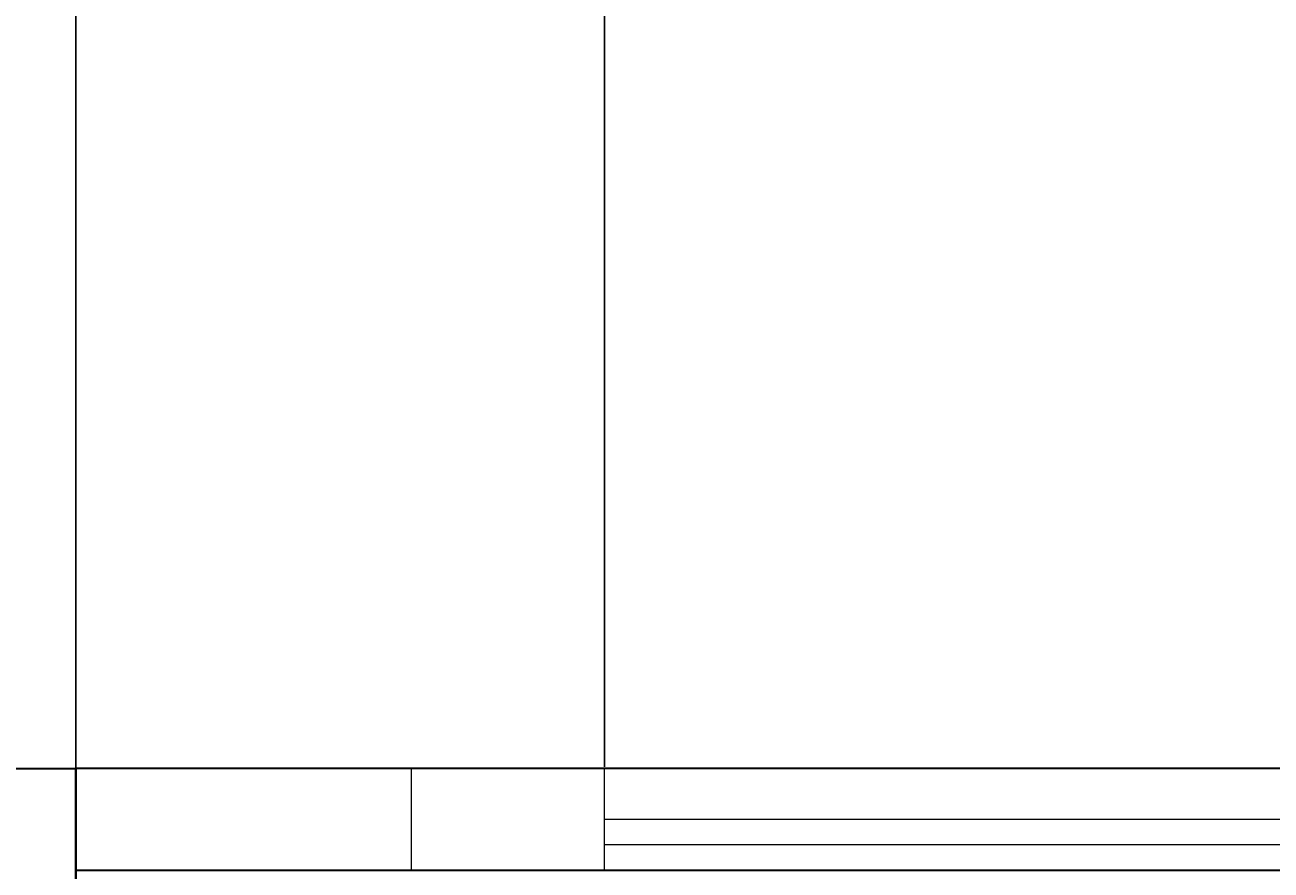
# Model space of a CAD drawing. Units: feet. Extents: x 105 to 1094, y -88 to 588.
# Tile 46 of 59: x 551 to 600, y 437 to 470. Entities that reach past the tile are written whole.
import ezdxf

# ---------------------------------------------------------------- set-up
doc = ezdxf.new("R2010")
doc.units = ezdxf.units.FT
doc.header["$MEASUREMENT"] = 0
for name, color, linetype, lineweight in [('A-ANNO-DIMS', 2, 'Continuous', 18), ('A-FLOR-PROJ', 8, 'Continuous', 25), ('A-GLAZ', 4, 'Continuous', 18), ('A-WALL', 7, 'Continuous', 35)]:
    doc.layers.add(name, color=color, linetype=linetype, lineweight=lineweight)
doc.styles.get("Standard").update_dxf_attribs({"font": 'arial.ttf'})
doc.dimstyles.get("Standard").update_dxf_attribs({"dimtxt": 0.18, "dimasz": 0.18, "dimexe": 0.18, "dimexo": 0.0625, "dimgap": 0.09, "dimtad": 0, "dimtih": 1, "dimtoh": 1, "dimdec": 4, "dimzin": 0, "dimdsep": 46, "dimtxsty": 'Standard', "dimcen": 0.09, "dimadec": 0, "dimazin": 0, "dimtfac": 1, "dimtdec": 4, "dimtofl": 0, "dimtmove": 0, "dimatfit": 3, "dimfxl": 1, "dimtolj": 1, "dimtzin": 0, "dimarcsym": 0})

# ---------------------------------------------------------------- blocks, each defined once
blk = doc.blocks.new('*D21')
at = {"layer": 'A-ANNO-DIMS', "color": 0, "lineweight": -2, "transparency": 16777216}
for p, q in [((849.626, 543.081), (105.458, 543.081)), ((105.638, 542.901), (105.638, 250.263)), ((105.638, -42.739), (105.638, 249.899)), ((849.626, -42.919), (105.458, -42.919))]:
    blk.add_line(p, q, dxfattribs=at)
at = {"layer": 'A-ANNO-DIMS', "color": 0, "transparency": 16777216}
for points in [[(105.608, 542.901), (105.668, 542.901), (105.638, 543.081)], [(105.608, -42.739), (105.668, -42.739), (105.638, -42.919)]]:
    blk.add_solid(points, dxfattribs=at)
at = {"layer": 'Defpoints', "color": 0, "transparency": 16777216}
for p in [(105.638, 543.081), (849.688, 543.081), (849.688, -42.919)]:
    blk.add_point(p, dxfattribs=at)
at = {"layer": 'A-ANNO-DIMS', "color": 0, "transparency": 16777216, "insert": (105.638, 250.081), "char_height": 0.18, "attachment_point": 5}
blk.add_mtext('\\A1;586', dxfattribs=at)
blk = doc.blocks.new('*D32')
at = {"layer": 'A-ANNO-DIMS', "color": 0, "lineweight": -2, "transparency": 16777216}
for p, q in [((646.626, 471.081), (105.458, 471.081)), ((105.638, 470.901), (105.638, 456.263)), ((105.638, 441.261), (105.638, 455.899)), ((646.626, 441.081), (105.458, 441.081))]:
    blk.add_line(p, q, dxfattribs=at)
at = {"layer": 'A-ANNO-DIMS', "color": 0, "transparency": 16777216}
for points in [[(105.608, 470.901), (105.668, 470.901), (105.638, 471.081)], [(105.608, 441.261), (105.668, 441.261), (105.638, 441.081)]]:
    blk.add_solid(points, dxfattribs=at)
at = {"layer": 'Defpoints', "color": 0, "transparency": 16777216}
for p in [(105.638, 471.081), (646.688, 471.081), (646.688, 441.081)]:
    blk.add_point(p, dxfattribs=at)
at = {"layer": 'A-ANNO-DIMS', "color": 0, "transparency": 16777216, "insert": (105.638, 456.081), "char_height": 0.18, "attachment_point": 5}
blk.add_mtext('\\A1;30', dxfattribs=at)
blk = doc.blocks.new('*D47')
at = {"layer": 'A-ANNO-DIMS', "color": 0, "lineweight": -2, "transparency": 16777216}
for p, q in [((552.688, 441.144), (552.688, 588.311)), ((552.868, 588.131), (562.621, 588.131)), ((573.303, 588.131), (563.55, 588.131)), ((573.483, 441.144), (573.483, 588.311))]:
    blk.add_line(p, q, dxfattribs=at)
at = {"layer": 'A-ANNO-DIMS', "color": 0, "transparency": 16777216}
for points in [[(552.868, 588.161), (552.868, 588.101), (552.688, 588.131)], [(573.303, 588.161), (573.303, 588.101), (573.483, 588.131)]]:
    blk.add_solid(points, dxfattribs=at)
at = {"layer": 'Defpoints', "color": 0, "transparency": 16777216}
for p in [(573.483, 588.131), (552.688, 441.081), (573.483, 441.081)]:
    blk.add_point(p, dxfattribs=at)
at = {"layer": 'A-ANNO-DIMS', "color": 0, "transparency": 16777216, "insert": (563.085, 588.131), "char_height": 0.18, "attachment_point": 5}
blk.add_mtext('\\A1;20.794', dxfattribs=at)
blk = doc.blocks.new('*D48')
at = {"layer": 'A-ANNO-DIMS', "color": 0, "lineweight": -2, "transparency": 16777216}
for p, q in [((573.483, 441.144), (573.483, 588.311)), ((573.663, 588.131), (603.263, 588.131)), ((633.303, 588.131), (603.702, 588.131)), ((633.483, 441.144), (633.483, 588.311))]:
    blk.add_line(p, q, dxfattribs=at)
at = {"layer": 'A-ANNO-DIMS', "color": 0, "transparency": 16777216}
for points in [[(573.663, 588.161), (573.663, 588.101), (573.483, 588.131)], [(633.303, 588.161), (633.303, 588.101), (633.483, 588.131)]]:
    blk.add_solid(points, dxfattribs=at)
at = {"layer": 'Defpoints', "color": 0, "transparency": 16777216}
for p in [(633.483, 588.131), (573.483, 441.081), (633.483, 441.081)]:
    blk.add_point(p, dxfattribs=at)
at = {"layer": 'A-ANNO-DIMS', "color": 0, "transparency": 16777216, "insert": (603.483, 588.131), "char_height": 0.18, "attachment_point": 5}
blk.add_mtext('\\A1;60', dxfattribs=at)

msp = doc.modelspace()

# ---------------------------------------------------------------- linework, layer by layer
at = {"layer": 'A-FLOR-PROJ'}
msp.add_line((552.6883, 471.0812), (552.6883, 441.0812), dxfattribs=at)
at = {"layer": 'A-GLAZ'}
for p, q in [((565.8941, 437.0812), (565.8941, 441.0812)), ((573.4826, 437.0812), (573.4826, 441.0812)), ((573.4826, 439.0812), (633.4826, 439.0812)), ((573.4826, 438.0812), (603.4826, 438.0812))]:
    msp.add_line(p, q, dxfattribs=at)
at = {"layer": 'A-WALL'}
for p, q in [((438.6883, 441.0812), (552.6883, 441.0812)), ((552.6883, 295.0812), (552.6883, 441.0812)), ((646.6883, 441.0812), (552.6883, 441.0812)), ((552.6883, 441.0812), (552.6883, 288.0812)), ((552.6883, 437.0812), (602.6883, 437.0812))]:
    msp.add_line(p, q, dxfattribs=at)

# ---------------------------------------------------------------- dimensions: what is measured, and where the dimension line sits
at = {"layer": 'A-ANNO-DIMS'}
for base, p1, p2, override, picture, middle in [((573.4826, 588.1312), (552.6883, 441.0812), (573.4826, 441.0812), {"dimdec": 3, "dimlfac": 1, "dimrnd": 0, "dimzin": 0, "dimdsep": 46, "dimlunit": 2}, '*D47', (563.0854, 588.1312)), ((633.4826, 588.1312), (573.4826, 441.0812), (633.4826, 441.0812), {"dimdec": 0, "dimlfac": 1, "dimrnd": 0, "dimzin": 0, "dimdsep": 46, "dimlunit": 2}, '*D48', (603.4826, 588.1312))]:
    dim = msp.add_linear_dim(base=base, p1=p1, p2=p2, dimstyle='Standard', override=override, dxfattribs=at)
    dim.commit()
    dim.dimension.update_dxf_attribs({"geometry": picture, "text_midpoint": middle})
for base, p1, p2, picture, middle in [((105.6383, 543.0812), (849.6883, -42.9188), (849.6883, 543.0812), '*D21', (105.6383, 250.0812)), ((105.6383, 471.0812), (646.6883, 441.0812), (646.6883, 471.0812), '*D32', (105.6383, 456.0812))]:
    dim = msp.add_linear_dim(base=base, p1=p1, p2=p2, angle=90, dimstyle='Standard', override={"dimdec": 0, "dimlfac": 1, "dimrnd": 0, "dimzin": 0, "dimdsep": 46, "dimlunit": 2}, dxfattribs=at)
    dim.commit()
    dim.dimension.update_dxf_attribs({"geometry": picture, "text_midpoint": middle})

doc.saveas('drawing.dxf')
